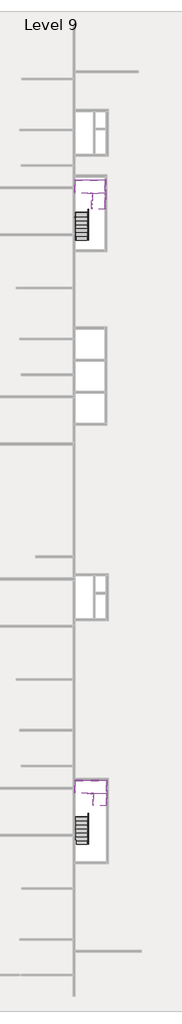
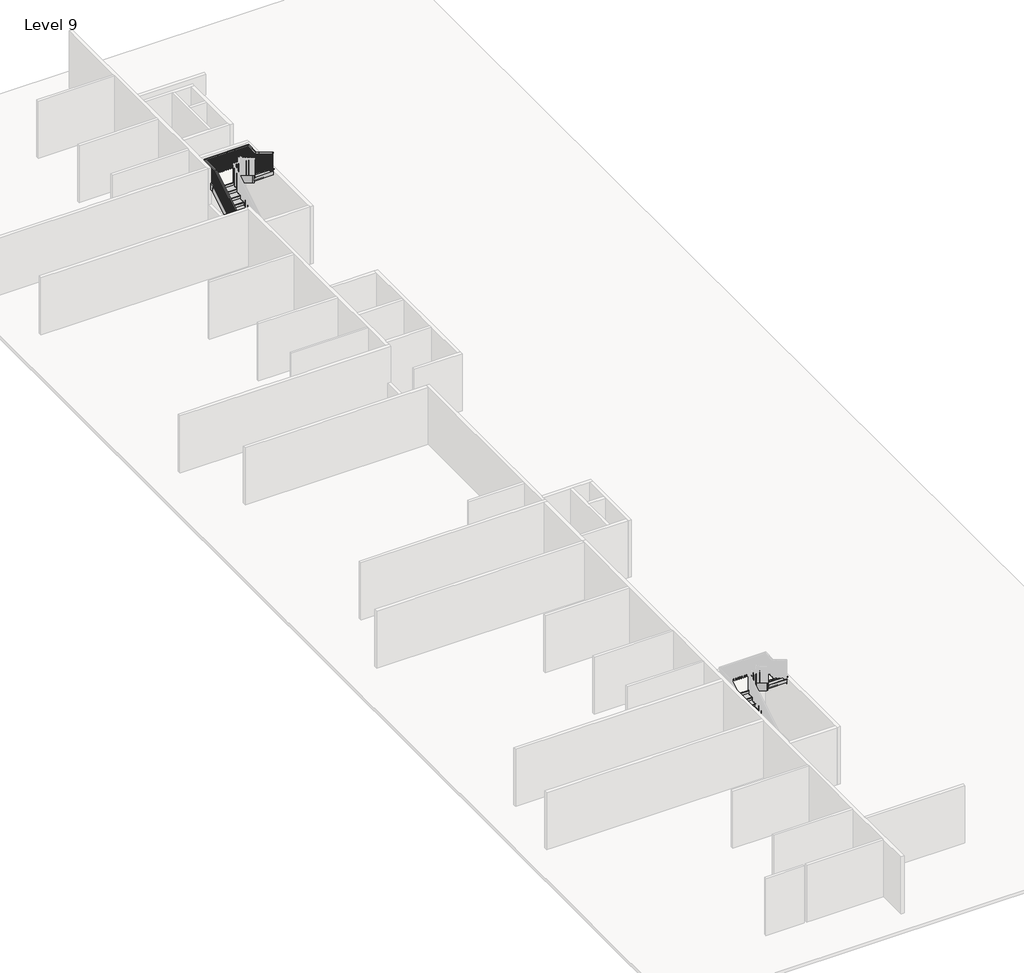
# One storey, part 8 of 8: 16 members, 4 stair flights, 2 slabs, 1 railing.
"""IFC4 building model written with IfcOpenShell, lengths in millimetres."""

from ifc_helpers import new_model, si_unit, frame, origin, place, context, project, spatial, polyline, outline, extrude, faceted_brep, transform, mapped, element, save
from components import non_monolithic_landing_15cb0957, non_monolithic_landing_50a26f39, stair_flight_ec606b3e, stair_flight_e995ea23, stair_flight_fc83273d, stair_flight_57f2103d

model = new_model("IFC4")

# Units and contexts
model_context = context("Model", 3, world=origin())
ifc_project = project(units=[si_unit("LENGTHUNIT", "METRE", prefix="MILLI")], contexts=[model_context])

# Site, building, storey
site = spatial("IfcSite", under=ifc_project)
building = spatial("IfcBuilding", under=site)
storey = spatial("IfcBuildingStorey", under=building, Name="Level 9", Elevation=49618.6172466)

# Members
placement = place(None, origin())
element("IfcMember", 1, ObjectType="Stringer - 2\" Width", at=placement, inside=storey, context=model_context, shape_type="SweptSolid", body=[
    extrude(outline(polyline([(-23154.3851539, 49618.6172466), (-23154.3851539, 49830.7317586), (-19467.0440987, 52065.4839133), (-19381.8896422, 51760.6839133), (-22916.2996422, 49618.6172466), (-23154.3851539, 49618.6172466)])), frame((-3668.2415084, 0.0, 0.0), z_axis=(1.0, 0.0, 0.0), x_axis=(0.0, 1.0, 0.0)), (0.0, 0.0, 1.0), 50.8),
])
element("IfcMember", 2, ObjectType="Stringer - 2\" Width", at=placement, inside=storey, context=model_context, shape_type="SweptSolid", body=[
    extrude(outline(polyline([(-23154.3851539, 49618.6172466), (-23154.3851539, 49830.7317586), (-19572.9851539, 52001.2772131), (-19572.9851539, 51644.8684516), (-22916.2996422, 49618.6172466), (-23154.3851539, 49618.6172466)])), frame((-2703.0415084, 0.0, 0.0), z_axis=(1.0, 0.0, 0.0), x_axis=(0.0, 1.0, 0.0)), (0.0, 0.0, 1.0), 50.8),
])
element("IfcMember", 3, ObjectType="Stringer - 2\" Width", at=placement, inside=storey, context=model_context, shape_type="SweptSolid", body=[
    extrude(outline(polyline([(-19297.9262092, 52065.4839133), (-19383.0806657, 51760.6839133), (-20360.3851539, 52352.9896637), (-20360.3851539, 52709.3984252), (-19297.9262092, 52065.4839133)])), frame((-1382.2415084, 0.0, 0.0), z_axis=(1.0, 0.0, 0.0), x_axis=(0.0, 1.0, 0.0)), (0.0, 0.0, 1.0), 50.8),
])
element("IfcMember", 4, ObjectType="Stringer - 2\" Width", at=placement, inside=storey, context=model_context, shape_type="SweptSolid", body=[
    extrude(outline(polyline([(-19522.1851539, 52201.3984252), (-19522.1851539, 51844.9896637), (-20360.3851539, 52352.9896637), (-20360.3851539, 52709.3984252), (-19522.1851539, 52201.3984252)])), frame((-2347.4415084, 0.0, 0.0), z_axis=(1.0, 0.0, 0.0), x_axis=(0.0, 1.0, 0.0)), (0.0, 0.0, 1.0), 50.8),
])
element("IfcMember", 5, ObjectType="Stringer - 2\" Width", at=placement, inside=storey, context=model_context, shape_type="Brep", body=[
    faceted_brep([(-1382.2415084, -19297.9262092, 52065.4839133), (-1331.4415084, -19297.9262092, 52065.4839133), (-1331.4415084, -18556.9851539, 52065.4839133), (-1382.2415084, -18607.7851539, 52065.4839133), (-1382.2415084, -19383.0806657, 51760.6839133), (-1382.2415084, -18607.7851539, 51760.6839133), (-1331.4415084, -19383.0806657, 51760.6839133), (-1331.4415084, -18556.9851539, 51760.6839133)], [[[0, 1, 2, 3]], [[4, 0, 3, 5]], [[6, 4, 5, 7]], [[1, 6, 7, 2]], [[1, 0, 4, 6]], [[2, 7, 5, 3]]]),
])
element("IfcMember", 6, ObjectType="Stringer - 2\" Width", at=placement, inside=storey, context=model_context, shape_type="SweptSolid", body=[
    extrude(outline(polyline([(-1331.4415084, -18556.9851539), (-1382.2415084, -18607.7851539), (-3617.4415084, -18607.7851539), (-3668.2415084, -18556.9851539), (-1331.4415084, -18556.9851539)])), frame((0.0, 0.0, 51760.6839133), z_axis=(0.0, 0.0, 1.0), x_axis=(1.0, 0.0, 0.0)), (0.0, 0.0, 1.0), 304.8),
])
element("IfcMember", 7, ObjectType="Stringer - 2\" Width", at=placement, inside=storey, context=model_context, shape_type="Brep", body=[
    faceted_brep([(-3617.4415084, -18607.7851539, 52065.4839133), (-3668.2415084, -18556.9851539, 52065.4839133), (-3668.2415084, -19467.0440987, 52065.4839133), (-3617.4415084, -19467.0440987, 52065.4839133), (-3617.4415084, -18607.7851539, 51760.6839133), (-3617.4415084, -19381.8896422, 51760.6839133), (-3668.2415084, -18556.9851539, 51760.6839133), (-3668.2415084, -19381.8896422, 51760.6839133)], [[[0, 1, 2, 3]], [[4, 0, 3, 5]], [[6, 4, 5, 7]], [[1, 6, 7, 2]], [[1, 0, 4, 6]], [[2, 7, 5, 3]]]),
])
element("IfcMember", 8, ObjectType="Stringer - 2\" Width", at=placement, inside=storey, context=model_context, shape_type="SweptSolid", body=[
    extrude(outline(polyline([(-2703.0415084, -19572.9851539), (-2703.0415084, -19522.1851539), (-2347.4415084, -19522.1851539), (-2347.4415084, -19572.9851539), (-2703.0415084, -19572.9851539)])), frame((0.0, 0.0, 51760.6839133), z_axis=(0.0, 0.0, 1.0), x_axis=(1.0, 0.0, 0.0)), (0.0, 0.0, 1.0), 304.8),
])
element("IfcMember", 9, ObjectType="Stringer - 2\" Width", at=placement, inside=storey, context=model_context, shape_type="SweptSolid", body=[
    extrude(outline(polyline([(19841.9216096, 49618.6172466), (19841.9216096, 49830.7317586), (23249.8626649, 51896.1505799), (23335.0171214, 51591.3505799), (20080.0071214, 49618.6172466), (19841.9216096, 49618.6172466)])), frame((-3668.2415084, 0.0, 0.0), z_axis=(1.0, 0.0, 0.0), x_axis=(0.0, 1.0, 0.0)), (0.0, 0.0, 1.0), 50.8),
])
element("IfcMember", 10, ObjectType="Stringer - 2\" Width", at=placement, inside=storey, context=model_context, shape_type="SweptSolid", body=[
    extrude(outline(polyline([(19841.9216096, 49618.6172466), (19841.9216096, 49830.7317586), (23143.9216096, 51831.9438798), (23143.9216096, 51475.5351183), (20080.0071214, 49618.6172466), (19841.9216096, 49618.6172466)])), frame((-2703.0415084, 0.0, 0.0), z_axis=(1.0, 0.0, 0.0), x_axis=(0.0, 1.0, 0.0)), (0.0, 0.0, 1.0), 50.8),
])
element("IfcMember", 11, ObjectType="Stringer - 2\" Width", at=placement, inside=storey, context=model_context, shape_type="SweptSolid", body=[
    extrude(outline(polyline([(23418.9805543, 51896.1505799), (23333.8260978, 51591.3505799), (22077.1216096, 52352.9896637), (22077.1216096, 52709.3984252), (23418.9805543, 51896.1505799)])), frame((-1483.8415084, 0.0, 0.0), z_axis=(1.0, 0.0, 0.0), x_axis=(0.0, 1.0, 0.0)), (0.0, 0.0, 1.0), 50.8),
])
element("IfcMember", 12, ObjectType="Stringer - 2\" Width", at=placement, inside=storey, context=model_context, shape_type="SweptSolid", body=[
    extrude(outline(polyline([(23194.7216096, 52032.0650919), (23194.7216096, 51675.6563304), (22077.1216096, 52352.9896637), (22077.1216096, 52709.3984252), (23194.7216096, 52032.0650919)])), frame((-2449.0415084, 0.0, 0.0), z_axis=(1.0, 0.0, 0.0), x_axis=(0.0, 1.0, 0.0)), (0.0, 0.0, 1.0), 50.8),
])
element("IfcMember", 13, ObjectType="Stringer - 2\" Width", at=placement, inside=storey, context=model_context, shape_type="Brep", body=[
    faceted_brep([(-1483.8415084, 23418.9805543, 51896.1505799), (-1433.0415084, 23418.9805543, 51896.1505799), (-1433.0415084, 24159.9216096, 51896.1505799), (-1483.8415084, 24109.1216096, 51896.1505799), (-1483.8415084, 23333.8260978, 51591.3505799), (-1483.8415084, 24109.1216096, 51591.3505799), (-1433.0415084, 23333.8260978, 51591.3505799), (-1433.0415084, 24159.9216096, 51591.3505799)], [[[0, 1, 2, 3]], [[4, 0, 3, 5]], [[6, 4, 5, 7]], [[1, 6, 7, 2]], [[1, 0, 4, 6]], [[2, 7, 5, 3]]]),
])
element("IfcMember", 14, ObjectType="Stringer - 2\" Width", at=placement, inside=storey, context=model_context, shape_type="SweptSolid", body=[
    extrude(outline(polyline([(-1433.0415084, 24159.9216096), (-1483.8415084, 24109.1216096), (-3617.4415084, 24109.1216096), (-3668.2415084, 24159.9216096), (-1433.0415084, 24159.9216096)])), frame((0.0, 0.0, 51591.3505799), z_axis=(0.0, 0.0, 1.0), x_axis=(1.0, 0.0, 0.0)), (0.0, 0.0, 1.0), 304.8),
])
element("IfcMember", 15, ObjectType="Stringer - 2\" Width", at=placement, inside=storey, context=model_context, shape_type="Brep", body=[
    faceted_brep([(-3617.4415084, 24109.1216096, 51896.1505799), (-3668.2415084, 24159.9216096, 51896.1505799), (-3668.2415084, 23249.8626649, 51896.1505799), (-3617.4415084, 23249.8626649, 51896.1505799), (-3617.4415084, 24109.1216096, 51591.3505799), (-3617.4415084, 23335.0171214, 51591.3505799), (-3668.2415084, 24159.9216096, 51591.3505799), (-3668.2415084, 23335.0171214, 51591.3505799)], [[[0, 1, 2, 3]], [[4, 0, 3, 5]], [[6, 4, 5, 7]], [[1, 6, 7, 2]], [[1, 0, 4, 6]], [[2, 7, 5, 3]]]),
])
element("IfcMember", 16, ObjectType="Stringer - 2\" Width", at=placement, inside=storey, context=model_context, shape_type="SweptSolid", body=[
    extrude(outline(polyline([(-2703.0415084, 23143.9216096), (-2703.0415084, 23194.7216096), (-2449.0415084, 23194.7216096), (-2449.0415084, 23143.9216096), (-2703.0415084, 23143.9216096)])), frame((0.0, 0.0, 51591.3505799), z_axis=(0.0, 0.0, 1.0), x_axis=(1.0, 0.0, 0.0)), (0.0, 0.0, 1.0), 304.8),
])

# Railing
element("IfcRailing", 17, ObjectType="Handrail - Rectangular", at=placement, inside=storey, context=model_context, shape_type="SolidModel", body=[
    faceted_brep([(-3617.4415084, 19841.9216096, 50702.3505799), (-3617.4415084, 19841.9216096, 50642.9491197), (-3566.6415084, 19841.9216096, 50642.9491197), (-3566.6415084, 19841.9216096, 50702.3505799), (-3617.4415084, 23194.7216096, 52734.3505799), (-3617.4415084, 23208.914019, 52683.5505799), (-3566.6415084, 23208.914019, 52683.5505799), (-3566.6415084, 23194.7216096, 52734.3505799), (-3617.4415084, 24109.1216096, 52734.3505799), (-3617.4415084, 24109.1216096, 52683.5505799), (-3566.6415084, 24058.3216096, 52683.5505799), (-3566.6415084, 24058.3216096, 52734.3505799), (-1483.8415084, 24109.1216096, 52734.3505799), (-1483.8415084, 24109.1216096, 52683.5505799), (-1534.6415084, 24058.3216096, 52683.5505799), (-1534.6415084, 24058.3216096, 52734.3505799), (-1483.8415084, 23474.1216096, 52734.3505799), (-1483.8415084, 23459.9292002, 52683.5505799), (-1534.6415084, 23459.9292002, 52683.5505799), (-1534.6415084, 23474.1216096, 52734.3505799), (-1483.8415084, 23194.7216096, 52903.6839133), (-1483.8415084, 23168.3918824, 52860.2398634), (-1534.6415084, 23168.3918824, 52860.2398634), (-1534.6415084, 23194.7216096, 52903.6839133), (-1483.8415084, 22077.1216096, 53581.0172466), (-1534.6415084, 22077.1216096, 53581.0172466), (-1534.6415084, 22077.1216096, 53521.6157863), (-1483.8415084, 22077.1216096, 53521.6157863)], [[[0, 1, 2, 3]], [[1, 0, 4, 5]], [[2, 1, 5, 6]], [[3, 2, 6, 7]], [[0, 3, 7, 4]], [[5, 4, 8, 9]], [[6, 5, 9, 10]], [[7, 6, 10, 11]], [[4, 7, 11, 8]], [[9, 8, 12, 13]], [[10, 9, 13, 14]], [[11, 10, 14, 15]], [[8, 11, 15, 12]], [[13, 12, 16, 17]], [[14, 13, 17, 18]], [[15, 14, 18, 19]], [[12, 15, 19, 16]], [[17, 16, 20, 21]], [[18, 17, 21, 22]], [[19, 18, 22, 23]], [[16, 19, 23, 20]], [[24, 25, 26, 27]], [[21, 20, 24, 27]], [[22, 21, 27, 26]], [[23, 22, 26, 25]], [[20, 23, 25, 24]]]),
    extrude(outline(polyline([(22188.2466096, 53454.2673015), (22188.2466096, 52497.2839133), (22169.1966096, 52497.2839133), (22169.1966096, 53465.812756), (22188.2466096, 53454.2673015)])), frame((-1518.7665084, 0.0, 0.0), z_axis=(1.0, 0.0, 0.0), x_axis=(0.0, 1.0, 0.0)), (0.0, 0.0, 1.0), 19.05),
    extrude(outline(polyline([(22289.8466096, 53392.6915439), (22289.8466096, 52497.2839133), (22270.7966096, 52497.2839133), (22270.7966096, 53404.2369985), (22289.8466096, 53392.6915439)])), frame((-1518.7665084, 0.0, 0.0), z_axis=(1.0, 0.0, 0.0), x_axis=(0.0, 1.0, 0.0)), (0.0, 0.0, 1.0), 19.05),
    extrude(outline(polyline([(22391.4466096, 53331.1157863), (22391.4466096, 52327.9505799), (22372.3966096, 52327.9505799), (22372.3966096, 53342.6612409), (22391.4466096, 53331.1157863)])), frame((-1518.7665084, 0.0, 0.0), z_axis=(1.0, 0.0, 0.0), x_axis=(0.0, 1.0, 0.0)), (0.0, 0.0, 1.0), 19.05),
    extrude(outline(polyline([(22493.0466096, 53269.5400288), (22493.0466096, 52327.9505799), (22473.9966096, 52327.9505799), (22473.9966096, 53281.0854833), (22493.0466096, 53269.5400288)])), frame((-1518.7665084, 0.0, 0.0), z_axis=(1.0, 0.0, 0.0), x_axis=(0.0, 1.0, 0.0)), (0.0, 0.0, 1.0), 19.05),
    extrude(outline(polyline([(22594.6466096, 53207.9642712), (22594.6466096, 52327.9505799), (22575.5966096, 52327.9505799), (22575.5966096, 53219.5097257), (22594.6466096, 53207.9642712)])), frame((-1518.7665084, 0.0, 0.0), z_axis=(1.0, 0.0, 0.0), x_axis=(0.0, 1.0, 0.0)), (0.0, 0.0, 1.0), 19.05),
    extrude(outline(polyline([(22696.2466096, 53146.3885136), (22696.2466096, 52158.6172466), (22677.1966096, 52158.6172466), (22677.1966096, 53157.9339682), (22696.2466096, 53146.3885136)])), frame((-1518.7665084, 0.0, 0.0), z_axis=(1.0, 0.0, 0.0), x_axis=(0.0, 1.0, 0.0)), (0.0, 0.0, 1.0), 19.05),
    extrude(outline(polyline([(22797.8466096, 53084.812756), (22797.8466096, 52158.6172466), (22778.7966096, 52158.6172466), (22778.7966096, 53096.3582106), (22797.8466096, 53084.812756)])), frame((-1518.7665084, 0.0, 0.0), z_axis=(1.0, 0.0, 0.0), x_axis=(0.0, 1.0, 0.0)), (0.0, 0.0, 1.0), 19.05),
    extrude(outline(polyline([(22899.4466096, 53023.2369985), (22899.4466096, 52158.6172466), (22880.3966096, 52158.6172466), (22880.3966096, 53034.782453), (22899.4466096, 53023.2369985)])), frame((-1518.7665084, 0.0, 0.0), z_axis=(1.0, 0.0, 0.0), x_axis=(0.0, 1.0, 0.0)), (0.0, 0.0, 1.0), 19.05),
    extrude(outline(polyline([(23001.0466096, 52961.6612409), (23001.0466096, 51989.2839133), (22981.9966096, 51989.2839133), (22981.9966096, 52973.2066954), (23001.0466096, 52961.6612409)])), frame((-1518.7665084, 0.0, 0.0), z_axis=(1.0, 0.0, 0.0), x_axis=(0.0, 1.0, 0.0)), (0.0, 0.0, 1.0), 19.05),
    extrude(outline(polyline([(23102.6466096, 52900.0854833), (23102.6466096, 51989.2839133), (23083.5966096, 51989.2839133), (23083.5966096, 52911.6309379), (23102.6466096, 52900.0854833)])), frame((-1518.7665084, 0.0, 0.0), z_axis=(1.0, 0.0, 0.0), x_axis=(0.0, 1.0, 0.0)), (0.0, 0.0, 1.0), 19.05),
    extrude(outline(polyline([(23280.4466096, 52792.3279076), (23280.4466096, 51819.9505799), (23261.3966096, 51819.9505799), (23261.3966096, 52803.8733621), (23280.4466096, 52792.3279076)])), frame((-1518.7665084, 0.0, 0.0), z_axis=(1.0, 0.0, 0.0), x_axis=(0.0, 1.0, 0.0)), (0.0, 0.0, 1.0), 19.05),
    extrude(outline(polyline([(23382.0466096, 52730.75215), (23382.0466096, 51819.9505799), (23362.9966096, 51819.9505799), (23362.9966096, 52742.2976045), (23382.0466096, 52730.75215)])), frame((-1518.7665084, 0.0, 0.0), z_axis=(1.0, 0.0, 0.0), x_axis=(0.0, 1.0, 0.0)), (0.0, 0.0, 1.0), 19.05),
    extrude(outline(polyline([(-1499.7165084, 23483.6466096), (-1499.7165084, 23464.5966096), (-1518.7665084, 23464.5966096), (-1518.7665084, 23483.6466096), (-1499.7165084, 23483.6466096)])), frame((0.0, 0.0, 51819.9505799), z_axis=(0.0, 0.0, 1.0), x_axis=(1.0, 0.0, 0.0)), (0.0, 0.0, 1.0), 863.6),
    extrude(outline(polyline([(-1499.7165084, 23585.2466096), (-1499.7165084, 23566.1966096), (-1518.7665084, 23566.1966096), (-1518.7665084, 23585.2466096), (-1499.7165084, 23585.2466096)])), frame((0.0, 0.0, 51819.9505799), z_axis=(0.0, 0.0, 1.0), x_axis=(1.0, 0.0, 0.0)), (0.0, 0.0, 1.0), 863.6),
    extrude(outline(polyline([(-1499.7165084, 23686.8466096), (-1499.7165084, 23667.7966096), (-1518.7665084, 23667.7966096), (-1518.7665084, 23686.8466096), (-1499.7165084, 23686.8466096)])), frame((0.0, 0.0, 51819.9505799), z_axis=(0.0, 0.0, 1.0), x_axis=(1.0, 0.0, 0.0)), (0.0, 0.0, 1.0), 863.6),
    extrude(outline(polyline([(-1499.7165084, 23788.4466096), (-1499.7165084, 23769.3966096), (-1518.7665084, 23769.3966096), (-1518.7665084, 23788.4466096), (-1499.7165084, 23788.4466096)])), frame((0.0, 0.0, 51819.9505799), z_axis=(0.0, 0.0, 1.0), x_axis=(1.0, 0.0, 0.0)), (0.0, 0.0, 1.0), 863.6),
    extrude(outline(polyline([(-1499.7165084, 23890.0466096), (-1499.7165084, 23870.9966096), (-1518.7665084, 23870.9966096), (-1518.7665084, 23890.0466096), (-1499.7165084, 23890.0466096)])), frame((0.0, 0.0, 51819.9505799), z_axis=(0.0, 0.0, 1.0), x_axis=(1.0, 0.0, 0.0)), (0.0, 0.0, 1.0), 863.6),
    extrude(outline(polyline([(-1499.7165084, 23991.6466096), (-1499.7165084, 23972.5966096), (-1518.7665084, 23972.5966096), (-1518.7665084, 23991.6466096), (-1499.7165084, 23991.6466096)])), frame((0.0, 0.0, 51819.9505799), z_axis=(0.0, 0.0, 1.0), x_axis=(1.0, 0.0, 0.0)), (0.0, 0.0, 1.0), 863.6),
    extrude(outline(polyline([(-1569.5665084, 24093.2466096), (-1550.5165084, 24093.2466096), (-1550.5165084, 24074.1966096), (-1569.5665084, 24074.1966096), (-1569.5665084, 24093.2466096)])), frame((0.0, 0.0, 51819.9505799), z_axis=(0.0, 0.0, 1.0), x_axis=(1.0, 0.0, 0.0)), (0.0, 0.0, 1.0), 863.6),
    extrude(outline(polyline([(-1671.1665084, 24093.2466096), (-1652.1165084, 24093.2466096), (-1652.1165084, 24074.1966096), (-1671.1665084, 24074.1966096), (-1671.1665084, 24093.2466096)])), frame((0.0, 0.0, 51819.9505799), z_axis=(0.0, 0.0, 1.0), x_axis=(1.0, 0.0, 0.0)), (0.0, 0.0, 1.0), 863.6),
    extrude(outline(polyline([(-1772.7665084, 24093.2466096), (-1753.7165084, 24093.2466096), (-1753.7165084, 24074.1966096), (-1772.7665084, 24074.1966096), (-1772.7665084, 24093.2466096)])), frame((0.0, 0.0, 51819.9505799), z_axis=(0.0, 0.0, 1.0), x_axis=(1.0, 0.0, 0.0)), (0.0, 0.0, 1.0), 863.6),
    extrude(outline(polyline([(-1874.3665084, 24093.2466096), (-1855.3165084, 24093.2466096), (-1855.3165084, 24074.1966096), (-1874.3665084, 24074.1966096), (-1874.3665084, 24093.2466096)])), frame((0.0, 0.0, 51819.9505799), z_axis=(0.0, 0.0, 1.0), x_axis=(1.0, 0.0, 0.0)), (0.0, 0.0, 1.0), 863.6),
    extrude(outline(polyline([(-1975.9665084, 24093.2466096), (-1956.9165084, 24093.2466096), (-1956.9165084, 24074.1966096), (-1975.9665084, 24074.1966096), (-1975.9665084, 24093.2466096)])), frame((0.0, 0.0, 51819.9505799), z_axis=(0.0, 0.0, 1.0), x_axis=(1.0, 0.0, 0.0)), (0.0, 0.0, 1.0), 863.6),
    extrude(outline(polyline([(-2077.5665084, 24093.2466096), (-2058.5165084, 24093.2466096), (-2058.5165084, 24074.1966096), (-2077.5665084, 24074.1966096), (-2077.5665084, 24093.2466096)])), frame((0.0, 0.0, 51819.9505799), z_axis=(0.0, 0.0, 1.0), x_axis=(1.0, 0.0, 0.0)), (0.0, 0.0, 1.0), 863.6),
    extrude(outline(polyline([(-2179.1665084, 24093.2466096), (-2160.1165084, 24093.2466096), (-2160.1165084, 24074.1966096), (-2179.1665084, 24074.1966096), (-2179.1665084, 24093.2466096)])), frame((0.0, 0.0, 51819.9505799), z_axis=(0.0, 0.0, 1.0), x_axis=(1.0, 0.0, 0.0)), (0.0, 0.0, 1.0), 863.6),
    extrude(outline(polyline([(-2280.7665084, 24093.2466096), (-2261.7165084, 24093.2466096), (-2261.7165084, 24074.1966096), (-2280.7665084, 24074.1966096), (-2280.7665084, 24093.2466096)])), frame((0.0, 0.0, 51819.9505799), z_axis=(0.0, 0.0, 1.0), x_axis=(1.0, 0.0, 0.0)), (0.0, 0.0, 1.0), 863.6),
    extrude(outline(polyline([(-2382.3665084, 24093.2466096), (-2363.3165084, 24093.2466096), (-2363.3165084, 24074.1966096), (-2382.3665084, 24074.1966096), (-2382.3665084, 24093.2466096)])), frame((0.0, 0.0, 51819.9505799), z_axis=(0.0, 0.0, 1.0), x_axis=(1.0, 0.0, 0.0)), (0.0, 0.0, 1.0), 863.6),
    extrude(outline(polyline([(-2483.9665084, 24093.2466096), (-2464.9165084, 24093.2466096), (-2464.9165084, 24074.1966096), (-2483.9665084, 24074.1966096), (-2483.9665084, 24093.2466096)])), frame((0.0, 0.0, 51819.9505799), z_axis=(0.0, 0.0, 1.0), x_axis=(1.0, 0.0, 0.0)), (0.0, 0.0, 1.0), 863.6),
    extrude(outline(polyline([(-2585.5665084, 24093.2466096), (-2566.5165084, 24093.2466096), (-2566.5165084, 24074.1966096), (-2585.5665084, 24074.1966096), (-2585.5665084, 24093.2466096)])), frame((0.0, 0.0, 51819.9505799), z_axis=(0.0, 0.0, 1.0), x_axis=(1.0, 0.0, 0.0)), (0.0, 0.0, 1.0), 863.6),
    extrude(outline(polyline([(-2687.1665084, 24093.2466096), (-2668.1165084, 24093.2466096), (-2668.1165084, 24074.1966096), (-2687.1665084, 24074.1966096), (-2687.1665084, 24093.2466096)])), frame((0.0, 0.0, 51819.9505799), z_axis=(0.0, 0.0, 1.0), x_axis=(1.0, 0.0, 0.0)), (0.0, 0.0, 1.0), 863.6),
    extrude(outline(polyline([(-2788.7665084, 24093.2466096), (-2769.7165084, 24093.2466096), (-2769.7165084, 24074.1966096), (-2788.7665084, 24074.1966096), (-2788.7665084, 24093.2466096)])), frame((0.0, 0.0, 51819.9505799), z_axis=(0.0, 0.0, 1.0), x_axis=(1.0, 0.0, 0.0)), (0.0, 0.0, 1.0), 863.6),
    extrude(outline(polyline([(-2890.3665084, 24093.2466096), (-2871.3165084, 24093.2466096), (-2871.3165084, 24074.1966096), (-2890.3665084, 24074.1966096), (-2890.3665084, 24093.2466096)])), frame((0.0, 0.0, 51819.9505799), z_axis=(0.0, 0.0, 1.0), x_axis=(1.0, 0.0, 0.0)), (0.0, 0.0, 1.0), 863.6),
    extrude(outline(polyline([(-2991.9665084, 24093.2466096), (-2972.9165084, 24093.2466096), (-2972.9165084, 24074.1966096), (-2991.9665084, 24074.1966096), (-2991.9665084, 24093.2466096)])), frame((0.0, 0.0, 51819.9505799), z_axis=(0.0, 0.0, 1.0), x_axis=(1.0, 0.0, 0.0)), (0.0, 0.0, 1.0), 863.6),
    extrude(outline(polyline([(-3093.5665084, 24093.2466096), (-3074.5165084, 24093.2466096), (-3074.5165084, 24074.1966096), (-3093.5665084, 24074.1966096), (-3093.5665084, 24093.2466096)])), frame((0.0, 0.0, 51819.9505799), z_axis=(0.0, 0.0, 1.0), x_axis=(1.0, 0.0, 0.0)), (0.0, 0.0, 1.0), 863.6),
    extrude(outline(polyline([(-3195.1665084, 24093.2466096), (-3176.1165084, 24093.2466096), (-3176.1165084, 24074.1966096), (-3195.1665084, 24074.1966096), (-3195.1665084, 24093.2466096)])), frame((0.0, 0.0, 51819.9505799), z_axis=(0.0, 0.0, 1.0), x_axis=(1.0, 0.0, 0.0)), (0.0, 0.0, 1.0), 863.6),
    extrude(outline(polyline([(-3296.7665084, 24093.2466096), (-3277.7165084, 24093.2466096), (-3277.7165084, 24074.1966096), (-3296.7665084, 24074.1966096), (-3296.7665084, 24093.2466096)])), frame((0.0, 0.0, 51819.9505799), z_axis=(0.0, 0.0, 1.0), x_axis=(1.0, 0.0, 0.0)), (0.0, 0.0, 1.0), 863.6),
    extrude(outline(polyline([(-3398.3665084, 24093.2466096), (-3379.3165084, 24093.2466096), (-3379.3165084, 24074.1966096), (-3398.3665084, 24074.1966096), (-3398.3665084, 24093.2466096)])), frame((0.0, 0.0, 51819.9505799), z_axis=(0.0, 0.0, 1.0), x_axis=(1.0, 0.0, 0.0)), (0.0, 0.0, 1.0), 863.6),
    extrude(outline(polyline([(-3499.9665084, 24093.2466096), (-3480.9165084, 24093.2466096), (-3480.9165084, 24074.1966096), (-3499.9665084, 24074.1966096), (-3499.9665084, 24093.2466096)])), frame((0.0, 0.0, 51819.9505799), z_axis=(0.0, 0.0, 1.0), x_axis=(1.0, 0.0, 0.0)), (0.0, 0.0, 1.0), 863.6),
    extrude(outline(polyline([(-3601.5665084, 23997.9966096), (-3601.5665084, 24017.0466096), (-3582.5165084, 24017.0466096), (-3582.5165084, 23997.9966096), (-3601.5665084, 23997.9966096)])), frame((0.0, 0.0, 51819.9505799), z_axis=(0.0, 0.0, 1.0), x_axis=(1.0, 0.0, 0.0)), (0.0, 0.0, 1.0), 863.6),
    extrude(outline(polyline([(-3601.5665084, 23896.3966096), (-3601.5665084, 23915.4466096), (-3582.5165084, 23915.4466096), (-3582.5165084, 23896.3966096), (-3601.5665084, 23896.3966096)])), frame((0.0, 0.0, 51819.9505799), z_axis=(0.0, 0.0, 1.0), x_axis=(1.0, 0.0, 0.0)), (0.0, 0.0, 1.0), 863.6),
    extrude(outline(polyline([(-3601.5665084, 23794.7966096), (-3601.5665084, 23813.8466096), (-3582.5165084, 23813.8466096), (-3582.5165084, 23794.7966096), (-3601.5665084, 23794.7966096)])), frame((0.0, 0.0, 51819.9505799), z_axis=(0.0, 0.0, 1.0), x_axis=(1.0, 0.0, 0.0)), (0.0, 0.0, 1.0), 863.6),
    extrude(outline(polyline([(-3601.5665084, 23693.1966096), (-3601.5665084, 23712.2466096), (-3582.5165084, 23712.2466096), (-3582.5165084, 23693.1966096), (-3601.5665084, 23693.1966096)])), frame((0.0, 0.0, 51819.9505799), z_axis=(0.0, 0.0, 1.0), x_axis=(1.0, 0.0, 0.0)), (0.0, 0.0, 1.0), 863.6),
    extrude(outline(polyline([(-3601.5665084, 23591.5966096), (-3601.5665084, 23610.6466096), (-3582.5165084, 23610.6466096), (-3582.5165084, 23591.5966096), (-3601.5665084, 23591.5966096)])), frame((0.0, 0.0, 51819.9505799), z_axis=(0.0, 0.0, 1.0), x_axis=(1.0, 0.0, 0.0)), (0.0, 0.0, 1.0), 863.6),
    extrude(outline(polyline([(-3601.5665084, 23489.9966096), (-3601.5665084, 23509.0466096), (-3582.5165084, 23509.0466096), (-3582.5165084, 23489.9966096), (-3601.5665084, 23489.9966096)])), frame((0.0, 0.0, 51819.9505799), z_axis=(0.0, 0.0, 1.0), x_axis=(1.0, 0.0, 0.0)), (0.0, 0.0, 1.0), 863.6),
    extrude(outline(polyline([(-3601.5665084, 23388.3966096), (-3601.5665084, 23407.4466096), (-3582.5165084, 23407.4466096), (-3582.5165084, 23388.3966096), (-3601.5665084, 23388.3966096)])), frame((0.0, 0.0, 51819.9505799), z_axis=(0.0, 0.0, 1.0), x_axis=(1.0, 0.0, 0.0)), (0.0, 0.0, 1.0), 863.6),
    extrude(outline(polyline([(-3601.5665084, 23286.7966096), (-3601.5665084, 23305.8466096), (-3582.5165084, 23305.8466096), (-3582.5165084, 23286.7966096), (-3601.5665084, 23286.7966096)])), frame((0.0, 0.0, 51819.9505799), z_axis=(0.0, 0.0, 1.0), x_axis=(1.0, 0.0, 0.0)), (0.0, 0.0, 1.0), 863.6),
    extrude(outline(polyline([(23102.6466096, 52619.1460894), (23102.6466096, 51650.6172466), (23083.5966096, 51650.6172466), (23083.5966096, 52607.6006348), (23102.6466096, 52619.1460894)])), frame((-3601.5665084, 0.0, 0.0), z_axis=(1.0, 0.0, 0.0), x_axis=(0.0, 1.0, 0.0)), (0.0, 0.0, 1.0), 19.05),
    extrude(outline(polyline([(23001.0466096, 52557.5703318), (23001.0466096, 51650.6172466), (22981.9966096, 51650.6172466), (22981.9966096, 52546.0248773), (23001.0466096, 52557.5703318)])), frame((-3601.5665084, 0.0, 0.0), z_axis=(1.0, 0.0, 0.0), x_axis=(0.0, 1.0, 0.0)), (0.0, 0.0, 1.0), 19.05),
    extrude(outline(polyline([(22899.4466096, 52495.9945742), (22899.4466096, 51481.2839133), (22880.3966096, 51481.2839133), (22880.3966096, 52484.4491197), (22899.4466096, 52495.9945742)])), frame((-3601.5665084, 0.0, 0.0), z_axis=(1.0, 0.0, 0.0), x_axis=(0.0, 1.0, 0.0)), (0.0, 0.0, 1.0), 19.05),
    extrude(outline(polyline([(22797.8466096, 52434.4188166), (22797.8466096, 51481.2839133), (22778.7966096, 51481.2839133), (22778.7966096, 52422.8733621), (22797.8466096, 52434.4188166)])), frame((-3601.5665084, 0.0, 0.0), z_axis=(1.0, 0.0, 0.0), x_axis=(0.0, 1.0, 0.0)), (0.0, 0.0, 1.0), 19.05),
    extrude(outline(polyline([(22696.2466096, 52372.8430591), (22696.2466096, 51481.2839133), (22677.1966096, 51481.2839133), (22677.1966096, 52361.2976045), (22696.2466096, 52372.8430591)])), frame((-3601.5665084, 0.0, 0.0), z_axis=(1.0, 0.0, 0.0), x_axis=(0.0, 1.0, 0.0)), (0.0, 0.0, 1.0), 19.05),
    extrude(outline(polyline([(22594.6466096, 52311.2673015), (22594.6466096, 51311.9505799), (22575.5966096, 51311.9505799), (22575.5966096, 52299.721847), (22594.6466096, 52311.2673015)])), frame((-3601.5665084, 0.0, 0.0), z_axis=(1.0, 0.0, 0.0), x_axis=(0.0, 1.0, 0.0)), (0.0, 0.0, 1.0), 19.05),
    extrude(outline(polyline([(22493.0466096, 52249.6915439), (22493.0466096, 51311.9505799), (22473.9966096, 51311.9505799), (22473.9966096, 52238.1460894), (22493.0466096, 52249.6915439)])), frame((-3601.5665084, 0.0, 0.0), z_axis=(1.0, 0.0, 0.0), x_axis=(0.0, 1.0, 0.0)), (0.0, 0.0, 1.0), 19.05),
    extrude(outline(polyline([(22391.4466096, 52188.1157863), (22391.4466096, 51311.9505799), (22372.3966096, 51311.9505799), (22372.3966096, 52176.5703318), (22391.4466096, 52188.1157863)])), frame((-3601.5665084, 0.0, 0.0), z_axis=(1.0, 0.0, 0.0), x_axis=(0.0, 1.0, 0.0)), (0.0, 0.0, 1.0), 19.05),
    extrude(outline(polyline([(22289.8466096, 52126.5400288), (22289.8466096, 51142.6172466), (22270.7966096, 51142.6172466), (22270.7966096, 52114.9945742), (22289.8466096, 52126.5400288)])), frame((-3601.5665084, 0.0, 0.0), z_axis=(1.0, 0.0, 0.0), x_axis=(0.0, 1.0, 0.0)), (0.0, 0.0, 1.0), 19.05),
    extrude(outline(polyline([(22188.2466096, 52064.9642712), (22188.2466096, 51142.6172466), (22169.1966096, 51142.6172466), (22169.1966096, 52053.4188166), (22188.2466096, 52064.9642712)])), frame((-3601.5665084, 0.0, 0.0), z_axis=(1.0, 0.0, 0.0), x_axis=(0.0, 1.0, 0.0)), (0.0, 0.0, 1.0), 19.05),
    extrude(outline(polyline([(22086.6466096, 52003.3885136), (22086.6466096, 51142.6172466), (22067.5966096, 51142.6172466), (22067.5966096, 51991.8430591), (22086.6466096, 52003.3885136)])), frame((-3601.5665084, 0.0, 0.0), z_axis=(1.0, 0.0, 0.0), x_axis=(0.0, 1.0, 0.0)), (0.0, 0.0, 1.0), 19.05),
    extrude(outline(polyline([(21985.0466096, 51941.812756), (21985.0466096, 50973.2839133), (21965.9966096, 50973.2839133), (21965.9966096, 51930.2673015), (21985.0466096, 51941.812756)])), frame((-3601.5665084, 0.0, 0.0), z_axis=(1.0, 0.0, 0.0), x_axis=(0.0, 1.0, 0.0)), (0.0, 0.0, 1.0), 19.05),
    extrude(outline(polyline([(21883.4466096, 51880.2369985), (21883.4466096, 50973.2839133), (21864.3966096, 50973.2839133), (21864.3966096, 51868.6915439), (21883.4466096, 51880.2369985)])), frame((-3601.5665084, 0.0, 0.0), z_axis=(1.0, 0.0, 0.0), x_axis=(0.0, 1.0, 0.0)), (0.0, 0.0, 1.0), 19.05),
    extrude(outline(polyline([(21781.8466096, 51818.6612409), (21781.8466096, 50803.9505799), (21762.7966096, 50803.9505799), (21762.7966096, 51807.1157863), (21781.8466096, 51818.6612409)])), frame((-3601.5665084, 0.0, 0.0), z_axis=(1.0, 0.0, 0.0), x_axis=(0.0, 1.0, 0.0)), (0.0, 0.0, 1.0), 19.05),
    extrude(outline(polyline([(21680.2466096, 51757.0854833), (21680.2466096, 50803.9505799), (21661.1966096, 50803.9505799), (21661.1966096, 51745.5400288), (21680.2466096, 51757.0854833)])), frame((-3601.5665084, 0.0, 0.0), z_axis=(1.0, 0.0, 0.0), x_axis=(0.0, 1.0, 0.0)), (0.0, 0.0, 1.0), 19.05),
    extrude(outline(polyline([(21578.6466096, 51695.5097257), (21578.6466096, 50803.9505799), (21559.5966096, 50803.9505799), (21559.5966096, 51683.9642712), (21578.6466096, 51695.5097257)])), frame((-3601.5665084, 0.0, 0.0), z_axis=(1.0, 0.0, 0.0), x_axis=(0.0, 1.0, 0.0)), (0.0, 0.0, 1.0), 19.05),
    extrude(outline(polyline([(21477.0466096, 51633.9339682), (21477.0466096, 50634.6172466), (21457.9966096, 50634.6172466), (21457.9966096, 51622.3885136), (21477.0466096, 51633.9339682)])), frame((-3601.5665084, 0.0, 0.0), z_axis=(1.0, 0.0, 0.0), x_axis=(0.0, 1.0, 0.0)), (0.0, 0.0, 1.0), 19.05),
    extrude(outline(polyline([(21375.4466096, 51572.3582106), (21375.4466096, 50634.6172466), (21356.3966096, 50634.6172466), (21356.3966096, 51560.812756), (21375.4466096, 51572.3582106)])), frame((-3601.5665084, 0.0, 0.0), z_axis=(1.0, 0.0, 0.0), x_axis=(0.0, 1.0, 0.0)), (0.0, 0.0, 1.0), 19.05),
    extrude(outline(polyline([(21273.8466096, 51510.782453), (21273.8466096, 50634.6172466), (21254.7966096, 50634.6172466), (21254.7966096, 51499.2369985), (21273.8466096, 51510.782453)])), frame((-3601.5665084, 0.0, 0.0), z_axis=(1.0, 0.0, 0.0), x_axis=(0.0, 1.0, 0.0)), (0.0, 0.0, 1.0), 19.05),
    extrude(outline(polyline([(21172.2466096, 51449.2066954), (21172.2466096, 50465.2839133), (21153.1966096, 50465.2839133), (21153.1966096, 51437.6612409), (21172.2466096, 51449.2066954)])), frame((-3601.5665084, 0.0, 0.0), z_axis=(1.0, 0.0, 0.0), x_axis=(0.0, 1.0, 0.0)), (0.0, 0.0, 1.0), 19.05),
    extrude(outline(polyline([(21070.6466096, 51387.6309379), (21070.6466096, 50465.2839133), (21051.5966096, 50465.2839133), (21051.5966096, 51376.0854833), (21070.6466096, 51387.6309379)])), frame((-3601.5665084, 0.0, 0.0), z_axis=(1.0, 0.0, 0.0), x_axis=(0.0, 1.0, 0.0)), (0.0, 0.0, 1.0), 19.05),
    extrude(outline(polyline([(20969.0466096, 51326.0551803), (20969.0466096, 50465.2839133), (20949.9966096, 50465.2839133), (20949.9966096, 51314.5097257), (20969.0466096, 51326.0551803)])), frame((-3601.5665084, 0.0, 0.0), z_axis=(1.0, 0.0, 0.0), x_axis=(0.0, 1.0, 0.0)), (0.0, 0.0, 1.0), 19.05),
    extrude(outline(polyline([(20867.4466096, 51264.4794227), (20867.4466096, 50295.9505799), (20848.3966096, 50295.9505799), (20848.3966096, 51252.9339682), (20867.4466096, 51264.4794227)])), frame((-3601.5665084, 0.0, 0.0), z_axis=(1.0, 0.0, 0.0), x_axis=(0.0, 1.0, 0.0)), (0.0, 0.0, 1.0), 19.05),
    extrude(outline(polyline([(20765.8466096, 51202.9036651), (20765.8466096, 50295.9505799), (20746.7966096, 50295.9505799), (20746.7966096, 51191.3582106), (20765.8466096, 51202.9036651)])), frame((-3601.5665084, 0.0, 0.0), z_axis=(1.0, 0.0, 0.0), x_axis=(0.0, 1.0, 0.0)), (0.0, 0.0, 1.0), 19.05),
    extrude(outline(polyline([(20664.2466096, 51141.3279076), (20664.2466096, 50126.6172466), (20645.1966096, 50126.6172466), (20645.1966096, 51129.782453), (20664.2466096, 51141.3279076)])), frame((-3601.5665084, 0.0, 0.0), z_axis=(1.0, 0.0, 0.0), x_axis=(0.0, 1.0, 0.0)), (0.0, 0.0, 1.0), 19.05),
    extrude(outline(polyline([(20562.6466096, 51079.75215), (20562.6466096, 50126.6172466), (20543.5966096, 50126.6172466), (20543.5966096, 51068.2066954), (20562.6466096, 51079.75215)])), frame((-3601.5665084, 0.0, 0.0), z_axis=(1.0, 0.0, 0.0), x_axis=(0.0, 1.0, 0.0)), (0.0, 0.0, 1.0), 19.05),
    extrude(outline(polyline([(20461.0466096, 51018.1763924), (20461.0466096, 50126.6172466), (20441.9966096, 50126.6172466), (20441.9966096, 51006.6309379), (20461.0466096, 51018.1763924)])), frame((-3601.5665084, 0.0, 0.0), z_axis=(1.0, 0.0, 0.0), x_axis=(0.0, 1.0, 0.0)), (0.0, 0.0, 1.0), 19.05),
    extrude(outline(polyline([(20359.4466096, 50956.6006348), (20359.4466096, 49957.2839133), (20340.3966096, 49957.2839133), (20340.3966096, 50945.0551803), (20359.4466096, 50956.6006348)])), frame((-3601.5665084, 0.0, 0.0), z_axis=(1.0, 0.0, 0.0), x_axis=(0.0, 1.0, 0.0)), (0.0, 0.0, 1.0), 19.05),
    extrude(outline(polyline([(20257.8466096, 50895.0248773), (20257.8466096, 49957.2839133), (20238.7966096, 49957.2839133), (20238.7966096, 50883.4794227), (20257.8466096, 50895.0248773)])), frame((-3601.5665084, 0.0, 0.0), z_axis=(1.0, 0.0, 0.0), x_axis=(0.0, 1.0, 0.0)), (0.0, 0.0, 1.0), 19.05),
    extrude(outline(polyline([(20156.2466096, 50833.4491197), (20156.2466096, 49957.2839133), (20137.1966096, 49957.2839133), (20137.1966096, 50821.9036651), (20156.2466096, 50833.4491197)])), frame((-3601.5665084, 0.0, 0.0), z_axis=(1.0, 0.0, 0.0), x_axis=(0.0, 1.0, 0.0)), (0.0, 0.0, 1.0), 19.05),
    extrude(outline(polyline([(20054.6466096, 50771.8733621), (20054.6466096, 49787.9505799), (20035.5966096, 49787.9505799), (20035.5966096, 50760.3279076), (20054.6466096, 50771.8733621)])), frame((-3601.5665084, 0.0, 0.0), z_axis=(1.0, 0.0, 0.0), x_axis=(0.0, 1.0, 0.0)), (0.0, 0.0, 1.0), 19.05),
    extrude(outline(polyline([(19953.0466096, 50710.2976045), (19953.0466096, 49787.9505799), (19933.9966096, 49787.9505799), (19933.9966096, 50698.75215), (19953.0466096, 50710.2976045)])), frame((-3601.5665084, 0.0, 0.0), z_axis=(1.0, 0.0, 0.0), x_axis=(0.0, 1.0, 0.0)), (0.0, 0.0, 1.0), 19.05),
    extrude(outline(polyline([(23204.2466096, 52838.5097257), (23204.2466096, 51819.9505799), (23185.1966096, 51819.9505799), (23185.1966096, 52850.0551803), (23204.2466096, 52838.5097257)])), frame((-1518.7665084, 0.0, 0.0), z_axis=(1.0, 0.0, 0.0), x_axis=(0.0, 1.0, 0.0)), (0.0, 0.0, 1.0), 19.05),
    extrude(outline(polyline([(-1518.7665084, 24093.2466096), (-1499.7165084, 24093.2466096), (-1499.7165084, 24074.1966096), (-1518.7665084, 24074.1966096), (-1518.7665084, 24093.2466096)])), frame((0.0, 0.0, 51819.9505799), z_axis=(0.0, 0.0, 1.0), x_axis=(1.0, 0.0, 0.0)), (0.0, 0.0, 1.0), 863.6),
    extrude(outline(polyline([(-3601.5665084, 24074.1966096), (-3601.5665084, 24093.2466096), (-3582.5165084, 24093.2466096), (-3582.5165084, 24074.1966096), (-3601.5665084, 24074.1966096)])), frame((0.0, 0.0, 51819.9505799), z_axis=(0.0, 0.0, 1.0), x_axis=(1.0, 0.0, 0.0)), (0.0, 0.0, 1.0), 863.6),
    extrude(outline(polyline([(23204.2466096, 52680.721847), (23204.2466096, 51819.9505799), (23185.1966096, 51819.9505799), (23185.1966096, 52669.1763924), (23204.2466096, 52680.721847)])), frame((-3601.5665084, 0.0, 0.0), z_axis=(1.0, 0.0, 0.0), x_axis=(0.0, 1.0, 0.0)), (0.0, 0.0, 1.0), 19.05),
    extrude(outline(polyline([(22096.1716096, 53510.0703318), (22096.1716096, 52497.2839133), (22077.1216096, 52497.2839133), (22077.1216096, 53521.6157863), (22096.1716096, 53510.0703318)])), frame((-1518.7665084, 0.0, 0.0), z_axis=(1.0, 0.0, 0.0), x_axis=(0.0, 1.0, 0.0)), (0.0, 0.0, 1.0), 19.05),
    extrude(outline(polyline([(19860.9716096, 50654.4945742), (19860.9716096, 49787.9505799), (19841.9216096, 49787.9505799), (19841.9216096, 50642.9491197), (19860.9716096, 50654.4945742)])), frame((-3601.5665084, 0.0, 0.0), z_axis=(1.0, 0.0, 0.0), x_axis=(0.0, 1.0, 0.0)), (0.0, 0.0, 1.0), 19.05),
])

# Slabs
non_monolithic_landing_shape = non_monolithic_landing_15cb0957(model_context)
element("IfcSlab", 18, ObjectType="Non-Monolithic Landing", at=placement, inside=storey, context=model_context, shape_type="MappedRepresentation", body=[
    mapped(non_monolithic_landing_shape, transform((0.0, 0.0, 0.0), x_axis=(1.0, 0.0, 0.0), y_axis=(0.0, 1.0, 0.0), z_axis=(0.0, 0.0, 1.0))),
])
non_monolithic_landing_2_shape = non_monolithic_landing_50a26f39(model_context)
element("IfcSlab", 19, ObjectType="Non-Monolithic Landing", at=placement, inside=storey, context=model_context, shape_type="MappedRepresentation", body=[
    mapped(non_monolithic_landing_2_shape, transform((0.0, 0.0, 0.0), x_axis=(1.0, 0.0, 0.0), y_axis=(0.0, 1.0, 0.0), z_axis=(0.0, 0.0, 1.0))),
])

# Stair flights
stair_flight_shape = stair_flight_ec606b3e(model_context)
element("IfcStairFlight", 20, ObjectType="2\" Tread 1\" Nosing 1/4\" Riser", at=placement, inside=storey, context=model_context, shape_type="MappedRepresentation", body=[
    mapped(stair_flight_shape, transform((0.0, 0.0, 0.0), x_axis=(1.0, 0.0, 0.0), y_axis=(0.0, 1.0, 0.0), z_axis=(0.0, 0.0, 1.0))),
])
stair_flight_2_shape = stair_flight_e995ea23(model_context)
element("IfcStairFlight", 21, ObjectType="2\" Tread 1\" Nosing 1/4\" Riser", at=placement, inside=storey, context=model_context, shape_type="MappedRepresentation", body=[
    mapped(stair_flight_2_shape, transform((0.0, 0.0, 0.0), x_axis=(1.0, 0.0, 0.0), y_axis=(0.0, 1.0, 0.0), z_axis=(0.0, 0.0, 1.0))),
])
stair_flight_3_shape = stair_flight_fc83273d(model_context)
element("IfcStairFlight", 22, ObjectType="2\" Tread 1\" Nosing 1/4\" Riser", at=placement, inside=storey, context=model_context, shape_type="MappedRepresentation", body=[
    mapped(stair_flight_3_shape, transform((0.0, 0.0, 0.0), x_axis=(1.0, 0.0, 0.0), y_axis=(0.0, 1.0, 0.0), z_axis=(0.0, 0.0, 1.0))),
])
stair_flight_4_shape = stair_flight_57f2103d(model_context)
element("IfcStairFlight", 23, ObjectType="2\" Tread 1\" Nosing 1/4\" Riser", at=placement, inside=storey, context=model_context, shape_type="MappedRepresentation", body=[
    mapped(stair_flight_4_shape, transform((0.0, 0.0, 0.0), x_axis=(1.0, 0.0, 0.0), y_axis=(0.0, 1.0, 0.0), z_axis=(0.0, 0.0, 1.0))),
])

save(model, "model.ifc")

# Revit data of these elements
# Type "Handrail - Rectangular"
#   Assembly Code = "C2010400"
#   built-in parameter 1008612 = 0.0416667 (stored number, unit not read)
#   built-in parameter 1008611 = 0.0416667 (stored number, unit not read)
#   built-in parameter 1008609 = 0.333333 (stored number, unit not read)
#   built-in parameter 1008604 = 0.166667 (stored number, unit not read)
#   built-in parameter 1008603 = 0.166667 (stored number, unit not read)
#   Railing Height = 3' - 0"
#   built-in parameter 1008630 = 2
#   built-in parameter 1008610 = 2
#   built-in parameter 1008618 = Baluster - Square : 3/4"
# Elements 1, 2, 3, 4, 5, 6, 7, 8, 9, 10, 11, 12, 13, 14, 15, 16 (IfcMember, "Stringer - 2\" Width")
#   Phase Created = New Construction
# Element 17 (IfcRailing, "Handrail - Rectangular")
#   Phase Created = New Construction
# Elements 18, 19 (IfcSlab, "Non-Monolithic Landing")
#   Phase Created = New Construction
# Elements 20, 21, 22, 23 (IfcStairFlight, "2\" Tread 1\" Nosing 1/4\" Riser")
#   Phase Created = New Construction
